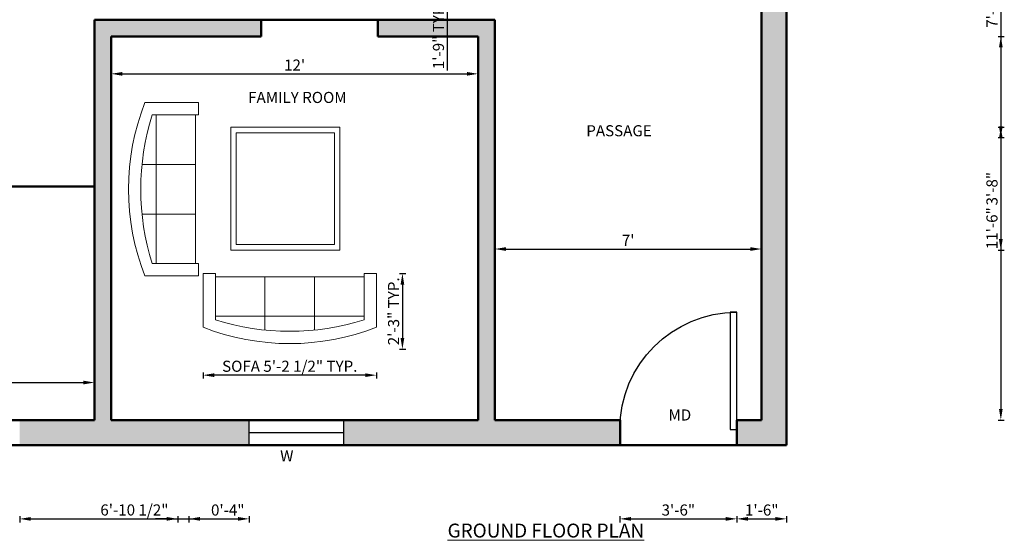
# Model space of a CAD drawing. Units: inches. Extents: x -31 to 511, y -453 to 49.
# Tile 3 of 4: x 157 to 511, y -453 to -265. Entities that reach past the tile are written whole.
import ezdxf

# ---------------------------------------------------------------- set-up
doc = ezdxf.new("R2010")
doc.units = ezdxf.units.IN
for name, color, linetype, lineweight in [('A-ANNO-DIMS', 2, 'Continuous', 18), ('A-ANNO-TEXT', 7, 'Continuous', 18), ('A-AREA-IDEN', 7, 'Continuous', 25), ('A-DOOR', 3, 'Continuous', 25), ('A-FURN', 8, 'Continuous', 18), ('A-GLAZ', 4, 'Continuous', 25), ('A-WALL', 7, 'Continuous', 50), ('A-WALL-PATT', 252, 'Continuous', 13)]:
    doc.layers.add(name, color=color, linetype=linetype, lineweight=lineweight)
doc.styles.get("Standard").update_dxf_attribs({"font": 'arial.ttf'})
doc.dimstyles.new('ISO-25', dxfattribs={"dimtxt": 4, "dimasz": 4, "dimexe": 1.25, "dimexo": 0.625, "dimtad": 1, "dimlunit": 3, "dimtxsty": 'Standard', "dimcen": 2.5, "dimadec": 0, "dimazin": 0, "dimtfac": 1, "dimtmove": 0, "dimatfit": 3, "dimfxl": 1, "dimfxlon": 1, "dimarcsym": 0})

# ---------------------------------------------------------------- blocks, each defined once
blk = doc.blocks.new('*U2')
for p, q in [((0, 0), (0, -100)), ((750, 0), (750, -100))]:
    blk.add_line(p, q)
blk.add_lwpolyline([(0, 0), (0, 750), (43.75, 750), (43.75, 0)], close=True)
blk.add_arc((0, 0), 750, 0, 90)
blk = doc.blocks.new('Sofa - Roundback 7 ft.')
for p, q in [((-12.00002, -32.4421), (-12.00003, -6.5971)), ((11.99997, -32.4421), (11.99998, -6.5971)), ((-36.000027, -34), (-36.000027, -11.4696)), ((-35.999844, -13.3819), (35.9998, -13.3819)), ((35.99998, -34), (35.99998, -11.4696)), ((-36.000027, -32.4421), (35.99998, -32.4421))]:
    blk.add_line(p, q)
for points in [[(-36.000027, -34), (-42.000027, -34), (-42.000027, -8)], [(41.99998, -8), (41.99998, -34), (35.99998, -34)]]:
    blk.add_lwpolyline(points)
for centre, radius, start, end in [((0, -114.25), 114.25, 68.43141, 111.5686), ((-0.00001, -127.1968), 121.1968, 72.72033, 107.2797)]:
    blk.add_arc(centre, radius, start, end)
blk = doc.blocks.new('*D23')
at = {"layer": 'A-ANNO-DIMS', "color": 0, "lineweight": -2, "transparency": 16777216}
for p, q in [((111.46, -396.89), (111.46, -394.64)), ((115.46, -395.89), (179.46, -395.89)), ((183.46, -396.89), (183.46, -394.64))]:
    blk.add_line(p, q, dxfattribs=at)
at = {"layer": 'A-ANNO-DIMS', "color": 0, "transparency": 16777216}
for points in [[(115.46, -395.23), (115.46, -396.56), (111.46, -395.89)], [(179.46, -395.23), (179.46, -396.56), (183.46, -395.89)]]:
    blk.add_solid(points, dxfattribs=at)
at = {"layer": 'Defpoints', "color": 0, "transparency": 16777216}
for p in [(183.46, -395.89), (111.46, -409.38), (183.46, -409.38)]:
    blk.add_point(p, dxfattribs=at)
at = {"layer": 'A-ANNO-DIMS', "color": 0, "transparency": 16777216, "insert": (147.46, -393.23), "char_height": 4, "attachment_point": 5}
blk.add_mtext("6'", dxfattribs=at)
blk = doc.blocks.new('*D24')
at = {"layer": 'A-ANNO-DIMS', "color": 0, "lineweight": -2, "transparency": 16777216}
for p, q in [((189.46, -283.85), (189.46, -286.1)), ((193.46, -284.85), (317.46, -284.85)), ((321.46, -283.85), (321.46, -286.1))]:
    blk.add_line(p, q, dxfattribs=at)
at = {"layer": 'A-ANNO-DIMS', "color": 0, "transparency": 16777216}
for points in [[(193.46, -284.19), (193.46, -285.52), (189.46, -284.85)], [(317.46, -284.19), (317.46, -285.52), (321.46, -284.85)]]:
    blk.add_solid(points, dxfattribs=at)
at = {"layer": 'Defpoints', "color": 0, "transparency": 16777216}
for p in [(189.46, -271.38), (321.46, -271.38), (321.46, -284.85)]:
    blk.add_point(p, dxfattribs=at)
at = {"layer": 'A-ANNO-DIMS', "color": 0, "transparency": 16777216, "insert": (255.46, -282.22), "char_height": 4, "attachment_point": 5}
blk.add_mtext("12'", dxfattribs=at)
blk = doc.blocks.new('*D25')
at = {"layer": 'A-ANNO-DIMS', "color": 0, "lineweight": -2, "transparency": 16777216}
for p, q in [((327.46, -348.87), (327.46, -346.62)), ((423.46, -348.87), (423.46, -346.62)), ((331.46, -347.87), (419.46, -347.87))]:
    blk.add_line(p, q, dxfattribs=at)
at = {"layer": 'A-ANNO-DIMS', "color": 0, "transparency": 16777216}
for points in [[(331.46, -347.2), (331.46, -348.53), (327.46, -347.87)], [(419.46, -347.2), (419.46, -348.53), (423.46, -347.87)]]:
    blk.add_solid(points, dxfattribs=at)
at = {"layer": 'Defpoints', "color": 0, "transparency": 16777216}
for p in [(423.46, -347.87), (327.46, -409.38), (423.46, -409.38)]:
    blk.add_point(p, dxfattribs=at)
at = {"layer": 'A-ANNO-DIMS', "color": 0, "transparency": 16777216, "insert": (375.46, -345.24), "char_height": 4, "attachment_point": 5}
blk.add_mtext("7'", dxfattribs=at)
blk = doc.blocks.new('WIN-34IN')
blk.add_line((0, 4.5), (34, 4.5))
blk.add_lwpolyline([(0, 9), (34, 9), (34, 0), (0, 0)], close=True)
blk = doc.blocks.new('*D36')
at = {"layer": 'A-ANNO-DIMS', "color": 0, "lineweight": -2, "transparency": 16777216}
for p, q in [((222.53, -392.24), (222.53, -394.49)), ((284.9, -392.24), (284.9, -394.49)), ((280.9, -393.24), (226.53, -393.24))]:
    blk.add_line(p, q, dxfattribs=at)
at = {"layer": 'A-ANNO-DIMS', "color": 0, "transparency": 16777216}
for points in [[(226.53, -392.57), (226.53, -393.91), (222.53, -393.24)], [(280.9, -392.57), (280.9, -393.91), (284.9, -393.24)]]:
    blk.add_solid(points, dxfattribs=at)
at = {"layer": 'Defpoints', "color": 0, "transparency": 16777216}
for p in [(222.53, -383.89), (284.9, -383.89), (222.53, -393.24)]:
    blk.add_point(p, dxfattribs=at)
at = {"layer": 'A-ANNO-DIMS', "color": 0, "transparency": 16777216, "insert": (253.72, -390.55), "char_height": 4, "attachment_point": 5}
blk.add_mtext('SOFA 5\'-2 1/2" TYP.', dxfattribs=at)
blk = doc.blocks.new('*D37')
at = {"layer": 'A-ANNO-DIMS', "color": 0, "lineweight": -2, "transparency": 16777216}
for p, q in [((293.26, -356.66), (295.51, -356.66)), ((294.26, -360.66), (294.26, -379.89)), ((293.26, -383.89), (295.51, -383.89))]:
    blk.add_line(p, q, dxfattribs=at)
at = {"layer": 'A-ANNO-DIMS', "color": 0, "transparency": 16777216}
for points in [[(293.59, -360.66), (294.92, -360.66), (294.26, -356.66)], [(293.59, -379.89), (294.92, -379.89), (294.26, -383.89)]]:
    blk.add_solid(points, dxfattribs=at)
at = {"layer": 'Defpoints', "color": 0, "transparency": 16777216}
for p in [(284.9, -356.66), (284.9, -383.89), (294.26, -383.89)]:
    blk.add_point(p, dxfattribs=at)
at = {"layer": 'A-ANNO-DIMS', "color": 0, "transparency": 16777216, "insert": (291.59, -370.27), "char_height": 4, "attachment_point": 5, "rotation": 90}
blk.add_mtext('2\'-3" TYP.', dxfattribs=at)
blk = doc.blocks.new('*D38')
at = {"layer": 'A-ANNO-DIMS', "color": 0, "lineweight": -2, "transparency": 16777216}
for p, q in [((270.85, -258.5), (270.85, -260.75)), ((305.24, -258.5), (305.24, -260.75)), ((270.85, -259.5), (197.91, -259.5)), ((301.24, -259.5), (274.85, -259.5))]:
    blk.add_line(p, q, dxfattribs=at)
at = {"layer": 'A-ANNO-DIMS', "color": 0, "transparency": 16777216}
for points in [[(274.85, -258.83), (274.85, -260.17), (270.85, -259.5)], [(301.24, -258.83), (301.24, -260.17), (305.24, -259.5)]]:
    blk.add_solid(points, dxfattribs=at)
at = {"layer": 'Defpoints', "color": 0, "transparency": 16777216}
for p in [(270.85, -254.34), (305.24, -254.34), (270.85, -259.5)]:
    blk.add_point(p, dxfattribs=at)
at = {"layer": 'A-ANNO-DIMS', "color": 0, "transparency": 16777216, "insert": (232.38, -256.8), "char_height": 4, "attachment_point": 5}
blk.add_mtext('LOVESEAT 2\'-10 1/2" TYP.', dxfattribs=at)
blk = doc.blocks.new('*D39')
at = {"layer": 'A-ANNO-DIMS', "color": 0, "lineweight": -2, "transparency": 16777216}
for p, q in [((309.4, -233.32), (311.65, -233.32)), ((310.4, -237.32), (310.4, -250.34)), ((309.4, -254.34), (311.65, -254.34)), ((310.4, -254.34), (310.4, -283.6))]:
    blk.add_line(p, q, dxfattribs=at)
at = {"layer": 'A-ANNO-DIMS', "color": 0, "transparency": 16777216}
for points in [[(309.73, -237.32), (311.06, -237.32), (310.4, -233.32)], [(309.73, -250.34), (311.06, -250.34), (310.4, -254.34)]]:
    blk.add_solid(points, dxfattribs=at)
at = {"layer": 'Defpoints', "color": 0, "transparency": 16777216}
for p in [(305.24, -233.32), (305.24, -254.34), (310.4, -254.34)]:
    blk.add_point(p, dxfattribs=at)
at = {"layer": 'A-ANNO-DIMS', "color": 0, "transparency": 16777216, "insert": (307.73, -270.97), "char_height": 4, "attachment_point": 5, "rotation": 90}
blk.add_mtext('1\'-9" TYP.', dxfattribs=at)
blk = doc.blocks.new('*D48')
at = {"layer": 'A-ANNO-DIMS', "color": 0, "lineweight": -2, "transparency": 16777216}
for p, q in [((508.55, -271.38), (510.8, -271.38)), ((509.55, -275.38), (509.55, -405.38)), ((508.55, -409.38), (510.8, -409.38))]:
    blk.add_line(p, q, dxfattribs=at)
at = {"layer": 'A-ANNO-DIMS', "color": 0, "transparency": 16777216}
for points in [[(508.88, -275.38), (510.22, -275.38), (509.55, -271.38)], [(508.88, -405.38), (510.22, -405.38), (509.55, -409.38)]]:
    blk.add_solid(points, dxfattribs=at)
at = {"layer": 'Defpoints', "color": 0, "transparency": 16777216}
for p in [(321.46, -271.38), (321.46, -409.38), (509.55, -409.38)]:
    blk.add_point(p, dxfattribs=at)
at = {"layer": 'A-ANNO-DIMS', "color": 0, "transparency": 16777216, "insert": (506.88, -340.38), "char_height": 4, "attachment_point": 5, "rotation": 90}
blk.add_mtext('11\'-6"', dxfattribs=at)
blk = doc.blocks.new('*D49')
at = {"layer": 'A-ANNO-DIMS', "color": 0, "lineweight": -2, "transparency": 16777216}
for p, q in [((372.45, -443.93), (372.45, -446.18)), ((376.45, -444.93), (410.6, -444.93)), ((414.6, -443.93), (414.6, -446.18))]:
    blk.add_line(p, q, dxfattribs=at)
at = {"layer": 'A-ANNO-DIMS', "color": 0, "transparency": 16777216}
for points in [[(376.45, -444.26), (376.45, -445.6), (372.45, -444.93)], [(410.6, -444.26), (410.6, -445.6), (414.6, -444.93)]]:
    blk.add_solid(points, dxfattribs=at)
at = {"layer": 'Defpoints', "color": 0, "transparency": 16777216}
for p in [(372.45, -418.38), (414.6, -418.38), (414.6, -444.93)]:
    blk.add_point(p, dxfattribs=at)
at = {"layer": 'A-ANNO-DIMS', "color": 0, "transparency": 16777216, "insert": (393.52, -442.26), "char_height": 4, "attachment_point": 5}
blk.add_mtext('3\'-6"', dxfattribs=at)
blk = doc.blocks.new('*D58')
at = {"layer": 'A-ANNO-DIMS', "color": 0, "lineweight": -2, "transparency": 16777216}
for p, q in [((508.55, -213.76), (510.8, -213.76)), ((509.55, -217.76), (509.55, -303.74)), ((508.55, -307.74), (510.8, -307.74))]:
    blk.add_line(p, q, dxfattribs=at)
at = {"layer": 'A-ANNO-DIMS', "color": 0, "transparency": 16777216}
for points in [[(508.88, -217.76), (510.22, -217.76), (509.55, -213.76)], [(508.88, -303.74), (510.22, -303.74), (509.55, -307.74)]]:
    blk.add_solid(points, dxfattribs=at)
at = {"layer": 'Defpoints', "color": 0, "transparency": 16777216}
for p in [(9.46, -213.76), (9.46, -307.74), (509.55, -307.74)]:
    blk.add_point(p, dxfattribs=at)
at = {"layer": 'A-ANNO-DIMS', "color": 0, "transparency": 16777216, "insert": (506.88, -260.75), "char_height": 4, "attachment_point": 5, "rotation": 90}
blk.add_mtext('7\'-10"', dxfattribs=at)
blk = doc.blocks.new('*D61')
at = {"layer": 'A-ANNO-DIMS', "color": 0, "lineweight": -2, "transparency": 16777216}
for p, q in [((156.55, -443.93), (156.55, -446.18)), ((160.55, -444.93), (235.1, -444.93)), ((239.1, -443.93), (239.1, -446.18))]:
    blk.add_line(p, q, dxfattribs=at)
at = {"layer": 'A-ANNO-DIMS', "color": 0, "transparency": 16777216}
for points in [[(160.55, -444.26), (160.55, -445.6), (156.55, -444.93)], [(235.1, -444.26), (235.1, -445.6), (239.1, -444.93)]]:
    blk.add_solid(points, dxfattribs=at)
at = {"layer": 'Defpoints', "color": 0, "transparency": 16777216}
for p in [(156.55, -418.38), (239.1, -418.38), (239.1, -444.93)]:
    blk.add_point(p, dxfattribs=at)
at = {"layer": 'A-ANNO-DIMS', "color": 0, "transparency": 16777216, "insert": (197.82, -442.24), "char_height": 4, "attachment_point": 5}
blk.add_mtext('6\'-10 1/2"', dxfattribs=at)
blk = doc.blocks.new('*D62')
at = {"layer": 'A-ANNO-DIMS', "color": 0, "lineweight": -2, "transparency": 16777216}
for p, q in [((414.6, -443.93), (414.6, -446.18)), ((418.6, -444.93), (428.46, -444.93)), ((432.46, -443.93), (432.46, -446.18))]:
    blk.add_line(p, q, dxfattribs=at)
at = {"layer": 'A-ANNO-DIMS', "color": 0, "transparency": 16777216}
for points in [[(418.6, -444.26), (418.6, -445.6), (414.6, -444.93)], [(428.46, -444.26), (428.46, -445.6), (432.46, -444.93)]]:
    blk.add_solid(points, dxfattribs=at)
at = {"layer": 'Defpoints', "color": 0, "transparency": 16777216}
for p in [(414.6, -418.38), (432.46, -418.38), (432.46, -444.93)]:
    blk.add_point(p, dxfattribs=at)
at = {"layer": 'A-ANNO-DIMS', "color": 0, "transparency": 16777216, "insert": (423.53, -442.26), "char_height": 4, "attachment_point": 5}
blk.add_mtext('1\'-6"', dxfattribs=at)
blk = doc.blocks.new('*D69')
at = {"layer": 'A-ANNO-DIMS', "color": 0, "lineweight": -2, "transparency": 16777216}
for p, q in [((232.48, 39.17), (232.48, 41.42)), ((236.48, 40.17), (267.79, 40.17)), ((271.79, 39.17), (271.79, 41.42))]:
    blk.add_line(p, q, dxfattribs=at)
at = {"layer": 'A-ANNO-DIMS', "color": 0, "transparency": 16777216}
for points in [[(236.48, 40.84), (236.48, 39.5), (232.48, 40.17)], [(267.79, 40.84), (267.79, 39.5), (271.79, 40.17)]]:
    blk.add_solid(points, dxfattribs=at)
at = {"layer": 'Defpoints', "color": 0, "transparency": 16777216}
for p in [(271.79, 40.17), (232.48, -304.06), (271.79, -304.06)]:
    blk.add_point(p, dxfattribs=at)
at = {"layer": 'A-ANNO-DIMS', "color": 0, "transparency": 16777216, "insert": (252.13, 42.86), "char_height": 4, "attachment_point": 5}
blk.add_mtext('3\'-3 1/2"', dxfattribs=at)
blk = doc.blocks.new('*D70')
at = {"layer": 'A-ANNO-DIMS', "color": 0, "lineweight": -2, "transparency": 16777216}
for p, q in [((508.55, -304.06), (510.8, -304.06)), ((509.55, -308.06), (509.55, -344.28)), ((508.55, -348.28), (510.8, -348.28))]:
    blk.add_line(p, q, dxfattribs=at)
at = {"layer": 'A-ANNO-DIMS', "color": 0, "transparency": 16777216}
for points in [[(508.88, -308.06), (510.22, -308.06), (509.55, -304.06)], [(508.88, -344.28), (510.22, -344.28), (509.55, -348.28)]]:
    blk.add_solid(points, dxfattribs=at)
at = {"layer": 'Defpoints', "color": 0, "transparency": 16777216}
for p in [(271.79, -304.06), (271.79, -348.28), (509.55, -348.28)]:
    blk.add_point(p, dxfattribs=at)
at = {"layer": 'A-ANNO-DIMS', "color": 0, "transparency": 16777216, "insert": (506.88, -326.17), "char_height": 4, "attachment_point": 5, "rotation": 90}
blk.add_mtext('3\'-8"', dxfattribs=at)
blk = doc.blocks.new('*D71')
at = {"layer": 'A-ANNO-DIMS', "color": 0, "lineweight": -2, "transparency": 16777216}
for p, q in [((209.46, -444.93), (205.46, -444.93)), ((213.46, -443.93), (213.46, -446.18)), ((213.46, -444.93), (217.46, -444.93)), ((217.46, -443.93), (217.46, -446.18)), ((221.46, -444.93), (237.35, -444.93))]:
    blk.add_line(p, q, dxfattribs=at)
at = {"layer": 'A-ANNO-DIMS', "color": 0, "transparency": 16777216}
for points in [[(209.46, -444.26), (209.46, -445.6), (213.46, -444.93)], [(221.46, -444.26), (221.46, -445.6), (217.46, -444.93)]]:
    blk.add_solid(points, dxfattribs=at)
at = {"layer": 'Defpoints', "color": 0, "transparency": 16777216}
for p in [(213.46, -139.38), (217.46, -139.38), (217.46, -444.93)]:
    blk.add_point(p, dxfattribs=at)
at = {"layer": 'A-ANNO-DIMS', "color": 0, "transparency": 16777216, "insert": (231.41, -442.26), "char_height": 4, "attachment_point": 5}
blk.add_mtext('0\'-4"', dxfattribs=at)

msp = doc.modelspace()

# ---------------------------------------------------------------- hatches: boundary and pattern name
at = {"layer": 'A-WALL-PATT'}
h = msp.add_hatch(color=256, dxfattribs=at)
h.dxf.hatch_style = 1
h.paths.add_polyline_path([(122.408, 13.62), (0.465, 13.62), (0.465, -55.742), (9.465, -55.742), (9.465, 4.62), (57.465, 4.62), (57.465, 0.62), (59.528, 0.62), (63.465, 0.62), (63.465, 4.62), (122.408, 4.62)])
h.paths.add_polyline_path([(267.569, 13.62), (156.408, 13.62), (156.408, 4.62), (207.465, 4.62), (207.465, -139.38), (203.465, -139.38), (203.465, -140.534), (203.465, -145.38), (217.465, -145.38), (217.465, -140.567), (217.465, -139.38), (213.465, -139.38), (213.465, 4.62), (267.569, 4.62)])
h.paths.add_polyline_path([(432.465, 13.62), (301.569, 13.62), (301.569, 4.62), (357.465, 4.62), (357.465, 0.312), (361.402, 0.312), (363.465, 0.312), (363.465, 4.62), (423.465, 4.62), (423.465, -55.742), (432.465, -55.742)])
h.paths.add_polyline_path([(432.465, -73.742), (423.465, -73.742), (423.465, -139.38), (363.465, -139.38), (363.465, -29.688), (357.465, -29.688), (357.465, -139.38), (253.542, -139.38, -0.0082235), (253.561, -140.567), (253.561, -145.38), (423.465, -145.38), (423.465, -409.38), (414.601, -409.38), (414.601, -412.759), (414.601, -418.38), (432.465, -418.38)])
h.paths.add_polyline_path([(167.12, -140.534, -0.00794), (167.139, -139.38), (63.465, -139.38), (63.465, -29.38), (57.465, -29.38), (57.465, -57.083), (57.472, -57.083), (57.472, -78.083), (57.465, -139.38), (9.465, -139.38), (9.465, -73.742), (0.465, -73.742), (0.465, -179.759), (9.465, -179.759), (9.465, -145.38), (167.12, -145.38)])
h.paths.add_polyline_path([(372.446, -412.759, -0.0200643), (372.581, -409.38), (327.465, -409.38), (327.465, -265.38), (285.454, -265.38), (285.454, -271.38), (321.465, -271.38), (321.465, -409.38), (273.096, -409.38), (273.096, -418.38), (372.446, -418.38)], flags=17)
h.paths.add_polyline_path([(239.096, -409.38), (189.465, -409.38), (189.465, -271.38), (243.454, -271.38), (243.454, -265.38), (183.465, -265.38), (183.465, -409.38), (156.552, -409.38), (156.552, -418.38), (239.096, -418.38)])
h.paths.add_polyline_path([(122.552, -409.38), (111.465, -409.38), (111.465, -325.38), (105.465, -325.38), (105.465, -409.38), (72.938, -409.38), (72.938, -418.38), (122.552, -418.38)])
h.paths.add_polyline_path([(38.938, -409.38), (9.465, -409.38), (9.465, -341.741), (0.465, -341.741), (0.465, -418.38), (38.938, -418.38)])
h.paths.add_polyline_path([(9.465, -213.759), (0.465, -213.759), (0.465, -307.741), (9.465, -307.741)])

# ---------------------------------------------------------------- linework, layer by layer
at = {"layer": 'A-FURN'}
for points in [[(232.479, -304.057), (271.786, -304.057), (271.786, -348.282), (232.479, -348.282)], [(234.479, -306.057), (269.786, -306.057), (269.786, -346.282), (234.479, -346.282)]]:
    msp.add_lwpolyline(points, close=True, dxfattribs=at)
at = {"layer": 'A-WALL'}
for p, q in [((432.465, 13.62), (432.465, -418.38)), ((423.465, -145.38), (423.465, -409.38)), ((183.465, -265.38), (183.465, -409.38)), ((183.465, -265.38), (327.465, -265.38)), ((243.454, -271.38), (243.454, -265.38)), ((285.454, -271.38), (285.454, -265.38)), ((327.465, -265.38), (327.465, -409.38)), ((189.465, -271.38), (243.454, -271.38)), ((189.465, -271.38), (189.465, -409.38)), ((285.454, -271.38), (321.465, -271.38)), ((321.465, -271.38), (321.465, -409.38)), ((105.465, -325.38), (183.465, -325.38)), ((183.465, -409.38), (111.465, -409.38)), ((321.465, -409.38), (189.465, -409.38)), ((372.601, -409.38), (327.465, -409.38)), ((372.601, -409.38), (372.601, -418.38)), ((423.465, -409.38), (414.601, -409.38)), ((414.601, -409.38), (414.601, -418.38)), ((432.465, -418.38), (0.465, -418.38))]:
    msp.add_line(p, q, dxfattribs=at)

# ---------------------------------------------------------------- block references
at = {"layer": 'A-DOOR', "xscale": -0.056207755241297, "yscale": 0.056207755241297, "zscale": 0.056207755241297}
msp.add_blockref('*U2', (414.601, -412.759), dxfattribs=at)
at = {"layer": 'A-FURN', "xscale": 0.7425074843458513, "yscale": 0.7425074843458513, "zscale": 0.7425074843458513}
for p, rotation in [((195.67, -326.362), 90), ((253.717, -381.905), 179.9999999999999)]:
    msp.add_blockref('Sofa - Roundback 7 ft.', p, dxfattribs=dict(at, rotation=rotation))
at = {"layer": 'A-GLAZ'}
msp.add_blockref('WIN-34IN', (239.097, -418.38), dxfattribs=at)

# ---------------------------------------------------------------- texts
at = {"layer": 'A-ANNO-TEXT', "attachment_point": 1}
for s, width, insert, char_height in [('MD', 13.88923, (389.973, -405.548), 4), ('W', 12.82281, (250.256, -420.292), 4), ('{\\fArial|b1|i0|c0|p34;\\LGROUND FLOOR PLAN}', 220.09768, (310.491, -446.64), 5)]:
    msp.add_mtext_dynamic_manual_height_columns(s, width=width, gutter_width=12.5, heights=[0], dxfattribs=dict(at, insert=insert, char_height=char_height))
at = {"layer": 'A-AREA-IDEN', "char_height": 4, "attachment_point": 1}
for s, width, insert in [('FAMILY ROOM', 59.57098, (238.744, -291.339)), ('PASSAGE', 69.90559, (360.399, -303.323))]:
    msp.add_mtext_dynamic_manual_height_columns(s, width=width, gutter_width=12.5, heights=[0], dxfattribs=dict(at, insert=insert))

# ---------------------------------------------------------------- dimensions: what is measured, and where the dimension line sits
at = {"layer": 'A-ANNO-DIMS'}
for base, p1, p2, override, picture, middle in [((271.786, 40.17), (232.479, -304.057), (271.786, -304.057), {"dimdec": 1, "dimlfac": 1, "dimrnd": 0, "dimzin": 1, "dimdsep": 46, "dimlunit": 4, "dimfrac": 2}, '*D69', (252.132, 42.865)), ((217.465, -444.93), (213.465, -139.38), (217.465, -139.38), {"dimdec": 1, "dimlfac": 1, "dimrnd": 0, "dimzin": 1, "dimdsep": 46, "dimlunit": 4, "dimfrac": 2}, '*D71', (231.406, -442.262)), ((183.465, -395.893), (111.465, -409.38), (183.465, -409.38), {"dimclrd": 0, "dimclre": 0, "dimclrt": 0}, '*D23', (147.465, -393.226)), ((239.096, -444.93), (156.552, -418.38), (239.096, -418.38), {"dimdec": 1, "dimlfac": 1, "dimrnd": 0, "dimzin": 1, "dimdsep": 46, "dimlunit": 4, "dimfrac": 2}, '*D61', (197.824, -442.237)), ((414.601, -444.93), (372.446, -418.38), (414.601, -418.38), {"dimdec": 1, "dimlfac": 1, "dimrnd": 0, "dimzin": 1, "dimdsep": 46, "dimlunit": 4, "dimfrac": 2}, '*D49', (393.524, -442.261)), ((432.465, -444.93), (414.601, -418.38), (432.465, -418.38), {"dimdec": 1, "dimlfac": 1, "dimrnd": 0, "dimzin": 1, "dimdsep": 46, "dimlunit": 4, "dimfrac": 2}, '*D62', (423.533, -442.262))]:
    dim = msp.add_linear_dim(base=base, p1=p1, p2=p2, dimstyle='ISO-25', override=override, dxfattribs=at)
    dim.commit()
    dim.dimension.update_dxf_attribs({"geometry": picture, "text_midpoint": middle})
for base, p1, p2, picture, middle in [((509.551, -307.741), (9.465, -213.759), (9.465, -307.741), '*D58', (506.883, -260.75)), ((509.551, -409.38), (321.465, -271.38), (321.465, -409.38), '*D48', (506.883, -340.38)), ((509.551, -348.282), (271.786, -304.057), (271.786, -348.282), '*D70', (506.882, -326.17))]:
    dim = msp.add_linear_dim(base=base, p1=p1, p2=p2, angle=90, dimstyle='ISO-25', override={"dimdec": 1, "dimlfac": 1, "dimrnd": 0, "dimzin": 1, "dimdsep": 46, "dimlunit": 4, "dimfrac": 2}, dxfattribs=at)
    dim.commit()
    dim.dimension.update_dxf_attribs({"geometry": picture, "text_midpoint": middle})
for base, p1, p2, angle, text, picture, middle in [((310.397, -254.34), (305.238, -233.324), (305.238, -254.34), 270, '<> TYP.', '*D39', (307.729, -270.968)), ((270.849, -259.498), (305.238, -254.34), (270.849, -254.34), 180, 'LOVESEAT <> TYP.', '*D38', (232.379, -256.804)), ((294.258, -383.885), (284.902, -356.66), (284.902, -383.885), 270, '<> TYP.', '*D37', (291.589, -370.273)), ((222.532, -393.241), (284.902, -383.885), (222.532, -383.885), 180, 'SOFA <> TYP.', '*D36', (253.717, -390.546))]:
    dim = msp.add_linear_dim(base=base, p1=p1, p2=p2, angle=angle, text=text, dimstyle='ISO-25', override={"dimdec": 1, "dimlfac": 1, "dimrnd": 0, "dimzin": 1, "dimdsep": 46, "dimlunit": 4, "dimfrac": 2}, dxfattribs=at)
    dim.commit()
    dim.dimension.update_dxf_attribs({"geometry": picture, "text_midpoint": middle})
for base, p1, p2, text, picture, middle in [((321.465, -284.853), (189.465, -271.38), (321.465, -271.38), "12'", '*D24', (255.465, -282.22)), ((423.465, -347.866), (327.465, -409.38), (423.465, -409.38), "7'", '*D25', (375.465, -345.241))]:
    dim = msp.add_linear_dim(base=base, p1=p1, p2=p2, text=text, dimstyle='ISO-25', override={"dimclrd": 0, "dimclre": 0, "dimclrt": 0}, dxfattribs=at)
    dim.commit()
    dim.dimension.update_dxf_attribs({"geometry": picture, "text_midpoint": middle})

doc.saveas('drawing.dxf')
